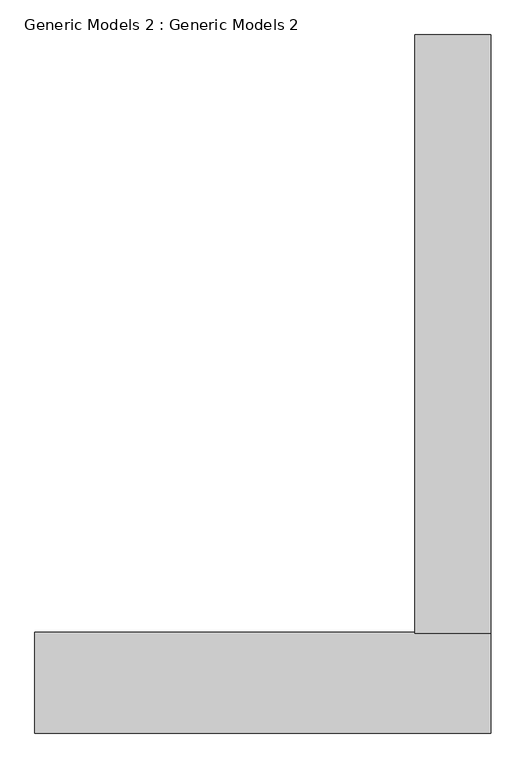
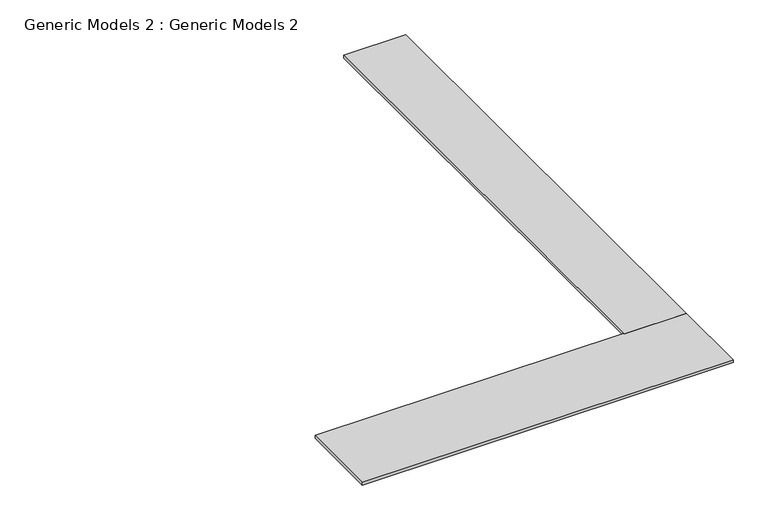
"""IFC4 building model written with IfcOpenShell, lengths in millimetres: proxy geometry, Generic Models 2 : Generic Models 2."""

from ifc_helpers import new_model, si_unit, frame, origin, place, context, project, spatial, polyline, outline, extrude, source, transform, mapped, element, save


def generic_models_2_generic_models_2_81f0c14a(model_context):
    return source(origin(), model_context, "Body", "SweptSolid", [
        extrude(outline(polyline([(6989.1654608, -10954.7822325), (6989.1654608, 16219.7563891), (10458.2200898, 16219.7563891), (10458.2200898, -10954.7822325), (6989.1654608, -10954.7822325)])), frame((0.0, 0.0, -152.4), z_axis=(0.0, 0.0, 1.0), x_axis=(1.0, 0.0, 0.0)), (0.0, 0.0, 1.0), 152.4),
        extrude(outline(polyline([(-10268.1799102, -10902.0843799), (10458.2200898, -10902.0843799), (10458.2200898, -15479.4436109), (-10268.1799102, -15479.4436109), (-10268.1799102, -10902.0843799)])), frame((0.0, 0.0, -152.4), z_axis=(0.0, 0.0, 1.0), x_axis=(1.0, 0.0, 0.0)), (0.0, 0.0, 1.0), 152.4),
    ])


if __name__ == "__main__":
    model = new_model("IFC4")
    model_context = context("Model", 3, world=origin())
    ifc_project = project(units=[si_unit("LENGTHUNIT", "METRE", prefix="MILLI")], contexts=[model_context])
    site = spatial("IfcSite", under=ifc_project)
    building = spatial("IfcBuilding", under=site)
    placement = place(None, origin())
    generic_models_2_generic_models_2_shape = generic_models_2_generic_models_2_81f0c14a(model_context)
    element("IfcBuildingElementProxy", 1, Name="Generic Models 2 : Generic Models 2", ObjectType="Generic Models 2 : Generic Models 2", at=placement, inside=building, context=model_context, shape_type="MappedRepresentation", body=[
        mapped(generic_models_2_generic_models_2_shape, transform((0.0, 0.0, 0.0), x_axis=(1.0, 0.0, 0.0), y_axis=(0.0, 1.0, 0.0), z_axis=(0.0, 0.0, 1.0))),
    ])
    save(model, "model.ifc")
